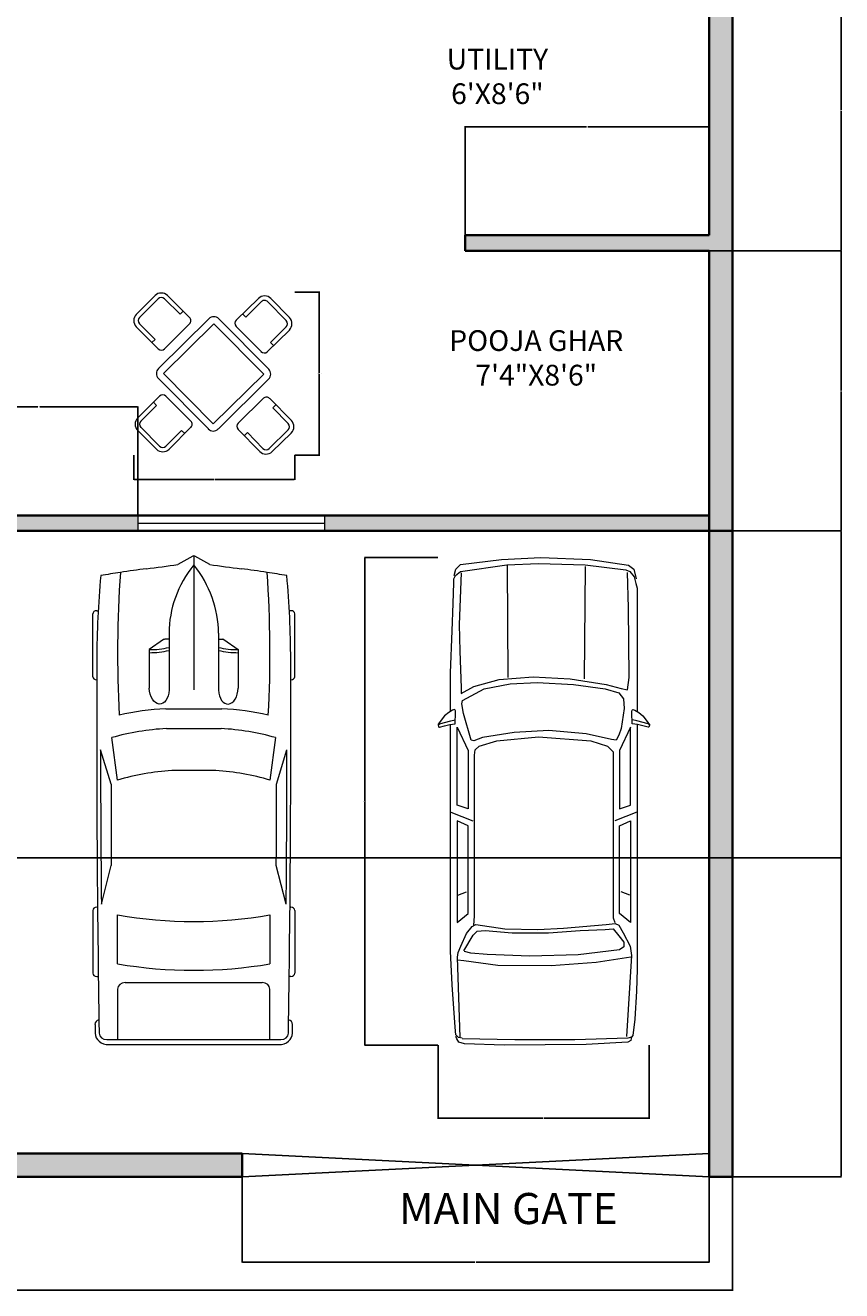
# Model space of a CAD drawing. Units: inches. Extents: x -89 to 661, y -827 to 77.
# Tile 3 of 5: x 347 to 661, y -827 to -339. Entities that reach past the tile are written whole.
import ezdxf

# ---------------------------------------------------------------- set-up
doc = ezdxf.new("R2010")
doc.units = ezdxf.units.IN
doc.header["$MEASUREMENT"] = 0
for name, color, linetype, lineweight in [('A-ANNO-DIMS', 2, 'Continuous', 18), ('A-ANNO-TEXT', 7, 'Continuous', 18), ('A-AREA-IDEN', 7, 'Continuous', 18), ('A-FURN', 34, 'Continuous', 18), ('A-GLAZ', 5, 'Continuous', 18), ('A-WALL', 7, 'Continuous', 35), ('A-WALL-PATT', 30, 'Continuous', 13), ('C-PRKG-VEHI', 5, 'Continuous', 13), ('L-GATE', 5, 'Continuous', 25)]:
    doc.layers.add(name, color=color, linetype=linetype, lineweight=lineweight)
doc.styles.get("Standard").update_dxf_attribs({"font": 'arial.ttf'})
doc.dimstyles.get("Standard").update_dxf_attribs({"dimtxt": 0.18, "dimasz": 0.18, "dimexe": 0.18, "dimexo": 0.0625, "dimgap": 0.09, "dimtad": 0, "dimtih": 1, "dimtoh": 1, "dimdec": 4, "dimzin": 0, "dimdsep": 46, "dimtxsty": 'Standard', "dimcen": 0.09, "dimadec": 0, "dimazin": 0, "dimtfac": 1, "dimtdec": 4, "dimtofl": 0, "dimtmove": 0, "dimatfit": 3, "dimfxl": 1, "dimtolj": 1, "dimtzin": 0, "dimarcsym": 0})

# ---------------------------------------------------------------- blocks, each defined once
blk = doc.blocks.new('*U2')
for p, q in [((21.1, 37.41), (21.1, 36.83)), ((46.55, 38.89), (22.35, 38.89)), ((47.8, 37.39), (47.8, 37.41)), ((87.99, 31.87), (74.76, 35.92)), ((134.31, 35.6), (119.29, 31.78)), ((135.45, 37.07), (135.45, 37.41)), ((136.7, 38.89), (160.9, 38.89)), ((162.15, 37.41), (162.15, 36.77)), ((70.03, 31.54), (86.41, 29.35)), ((138.42, 29.35), (157.25, 29.35)), ((186.47, 29.35), (167.01, 29.35)), ((186.47, -33.5), (186.47, 33.5)), ((188.4, -32.76), (188.4, 32.76)), ((164.52, 26.39), (164.52, -26.39)), ((32.27, 11.63), (36.13, 17.17)), ((36.13, 17.17), (50.94, 17.17)), ((32.12, 9.51), (32.12, 11.15)), ((58.92, -10.77), (58.92, 10.77)), ((66.55, -10.53), (66.55, 10.53)), ((186.47, -10.53), (186.47, 10.53)), ((3.27, 6.13), (0.1, 0.41)), ((29.77, 9.51), (51.68, 9.51)), ((82.74, 8.5), (82.74, -8.5)), ((0, 0), (51.68, 0)), ((0.1, -0.41), (3.27, -6.13)), ((29.77, -9.51), (51.68, -9.51)), ((32.12, -9.51), (32.12, -11.15)), ((32.27, -11.63), (36.13, -17.17)), ((36.13, -17.17), (50.94, -17.17)), ((86.41, -29.35), (70.03, -31.54)), ((87.99, -31.87), (74.76, -35.92)), ((134.31, -35.6), (119.29, -31.78)), ((157.25, -29.35), (138.42, -29.35)), ((167.01, -29.35), (186.47, -29.35)), ((21.1, -37.41), (21.1, -36.83)), ((46.55, -38.89), (22.35, -38.89)), ((47.8, -37.39), (47.8, -37.41)), ((135.45, -37.07), (135.45, -37.41)), ((136.7, -38.89), (160.9, -38.89)), ((162.15, -37.41), (162.15, -36.77))]:
    blk.add_line(p, q)
for centre, major_axis, ratio, start_param, end_param in [((266.03, -27.52), (0, 313.31), 0.842304, 1.367076, 1.39176), ((41.19, -490.86), (0, 528.23), 0.842304, 0.00281, 0.075598), ((22.35, 37.41), (0, -1.48), 0.842304, 3.141593, 4.712389), ((64.48, -10555.62), (0, 10593.03), 0.842304, -0.013397, 0.002797), ((46.55, 37.41), (0, 1.48), 0.842304, -1.570796, 0), ((64.48, -10555.62), (0, -10591.55), 0.842304, 3.133765, 3.140441), ((136.7, 37.41), (0, -1.48), 0.842304, 3.141593, 4.712389), ((160.9, 37.41), (0, 1.48), 0.842304, -1.570796, 0), ((180.63, 35.84), (0, 2.22), 0.842304, -0.013017, 1.249894), ((64.48, -10556.36), (0, 10595.31), 0.842304, -0.013397, -0.013017), ((183.98, 33.5), (0, -2.96), 0.842304, 1.570796, 3.128196), ((183.98, 32.76), (0, -5.25), 0.842304, 1.570796, 3.128196), ((37.47, -593.96), (0, -623.33), 0.842304, 3.096046, 3.200911), ((135.29, 5.39), (0, 81.77), 0.842304, 1.245306, 1.50788), ((149.6, 2.8), (0, -79.58), 0.842304, 4.372215, 4.640744), ((95.79, -3666.35), (0, -3698.24), 0.842304, 3.134049, 3.144098), ((17.08, 0), (0, 147.02), 0.842304, 4.511394, 4.913384), ((35.91, 0), (0, 147.02), 0.842304, 4.511394, 4.913384), ((167.01, 26.39), (0, 2.96), 0.842304, 0, 1.570796), ((259.18, -27.52), (0, -305.3), 0.842304, 4.528606, 4.561838), ((134.4, 5.39), (0, -89.78), 0.842304, 4.449482, 4.652344), ((-204.49, 52.4), (0, -250.96), 0.842304, 1.385369, 1.434372), ((13.04, 17.01), (0, 27.42), 0.842304, 4.435146, 4.718221), ((14.2, 17.01), (0, 27.42), 0.842304, 4.435146, 4.718221), ((50.79, 13.34), (6.34, -0.36), 0.603834, -1.395552, 1.581315), ((32.75, 11.15), (0, 0.74), 0.842304, 0.879714, 1.570796), ((29.77, -46.66), (0, 56.17), 0.842304, 0, 0.590319), ((0.62, 0), (0, -0.74), 0.842304, 4.131459, 5.293319), ((29.77, 46.66), (0, 56.17), 0.842304, 2.551274, 3.141593), ((-204.49, -52.4), (0, 250.96), 0.842304, -1.434372, -1.385369), ((13.04, -17.01), (0, -27.42), 0.842304, 1.564964, 1.848039), ((14.2, -17.01), (0, -27.42), 0.842304, 1.564964, 1.848039), ((149.6, -2.8), (0, -79.58), 0.842304, -1.499151, -1.230623), ((32.75, -11.15), (0, -0.74), 0.842304, 4.712389, 5.403472), ((134.4, -5.39), (0, -89.78), 0.842304, -1.510751, -1.307889), ((135.29, -5.39), (0, -81.77), 0.842304, -1.50788, -1.245306), ((259.18, 27.52), (0, 305.3), 0.842304, 1.721348, 1.754579), ((266.03, 27.52), (0, 313.31), 0.842304, 1.749832, 1.774517), ((37.47, 593.96), (0, -623.33), 0.842304, -0.059319, 0.045547), ((167.01, -26.39), (0, -2.96), 0.842304, 4.712389, 6.283185), ((95.79, 3666.35), (0, -3698.24), 0.842304, -0.002505, 0.007544), ((183.98, -33.5), (0, 2.96), 0.842304, 3.15499, 4.712389), ((183.98, -32.76), (0, -5.25), 0.842304, 0.013397, 1.570796), ((41.19, 490.86), (0, -528.23), 0.842304, -0.075598, -0.00281), ((22.35, -37.41), (0, 1.48), 0.842304, 1.570796, 3.141593), ((64.48, 10555.62), (0, 10593.03), 0.842304, 3.138796, 3.15499), ((46.55, -37.41), (0, -1.48), 0.842304, 0, 1.570796), ((64.48, 10555.62), (0, -10591.55), 0.842304, 0.001152, 0.007828), ((136.7, -37.41), (0, -1.48), 0.842304, -1.570796, 0), ((160.9, -37.41), (0, 1.48), 0.842304, 3.141593, 4.712389), ((180.63, -35.84), (0, -2.22), 0.842304, -1.249894, 0.013017), ((64.48, 10556.36), (0, 10595.31), 0.842304, 3.15461, 3.15499)]:
    blk.add_ellipse(centre, major_axis=major_axis, ratio=ratio, start_param=start_param, end_param=end_param)
at = {"extrusion": (0, 0, -1)}
blk.add_ellipse((50.79, -13.34), major_axis=(6.34, 0.36), ratio=0.603834, start_param=-1.395552, end_param=1.581315, dxfattribs=at)
blk = doc.blocks.new('A$C381B4D24')
for p, q in [((-0.244, 1.001), (-0.212, 1.042)), ((-0.212, 1.042), (-0.142, 1.096)), ((-0.133, 1.095), (-0.162, 0.981)), ((-0.142, 1.096), (-0.127, 1.108)), ((-0.12, 1.108), (-0.133, 1.095)), ((-0.127, 1.108), (-0.12, 1.108)), ((-0.11, 1.042), (-0.124, 0.989)), ((-0.119, 1.108), (-0.097, 1.101)), ((-0.097, 1.095), (-0.11, 1.042)), ((-0.097, 1.101), (-0.097, 1.095)), ((-1.777, 0.52), (-1.719, 0.898)), ((-1.719, 0.898), (-1.68, 0.953)), ((-1.68, 0.953), (-1.583, 0.977)), ((-1.672, 0.873), (-1.658, 0.914)), ((-1.658, 0.914), (-1.605, 0.955)), ((-1.293, 0.898), (-1.648, 0.89)), ((-1.605, 0.955), (-1.538, 0.971)), ((-1.538, 0.971), (-1.491, 0.987)), ((-1.491, 0.987), (-0.253, 0.987)), ((-0.596, 0.906), (-1.293, 0.898)), ((-0.473, 0.89), (-0.596, 0.906)), ((-0.486, 0.827), (-0.473, 0.89)), ((-0.274, 0.942), (-0.269, 0.963)), ((-0.269, 0.935), (-0.274, 0.942)), ((-0.269, 0.963), (-0.244, 1.001)), ((-0.263, 0.932), (-0.269, 0.935)), ((-0.246, 0.932), (-0.263, 0.932)), ((-0.131, 0.936), (-0.246, 0.932)), ((-0.162, 0.981), (-0.17, 0.938)), ((-0.128, 0.963), (-0.131, 0.936)), ((-0.124, 0.989), (-0.128, 0.963)), ((-0.124, 0.987), (2.324, 0.987)), ((0.682, 0.92), (-0.097, 0.92)), ((-0.097, 0.92), (0.136, 0.809)), ((0.721, 0.809), (0.682, 0.92)), ((0.753, 0.983), (0.838, 0.761)), ((0.838, 0.92), (1.857, 0.92)), ((0.89, 0.809), (0.838, 0.92)), ((1.585, 0.912), (1.552, 0.825)), ((1.857, 0.92), (1.766, 0.809)), ((1.961, 0.844), (2.095, 0.916)), ((2.095, 0.916), (2.188, 0.93)), ((2.188, 0.93), (2.998, 0.88)), ((2.206, 0.923), (2.258, 0.574)), ((2.324, 0.987), (2.546, 0.978)), ((2.546, 0.978), (2.826, 0.963)), ((2.826, 0.963), (2.989, 0.944)), ((2.989, 0.944), (3.007, 0.929)), ((2.998, 0.93), (3.039, 0.923)), ((3.007, 0.929), (3.015, 0.893)), ((3.015, 0.893), (3.033, 0.361)), ((3.039, 0.923), (3.056, 0.894)), ((3.056, 0.894), (3.08, 0.475)), ((-1.725, 0.465), (-1.672, 0.873)), ((-0.524, 0.677), (-0.486, 0.827)), ((-0.481, 0.666), (-0.442, 0.801)), ((-0.442, 0.801), (-0.383, 0.849)), ((-0.383, 0.849), (-0.286, 0.856)), ((-0.286, 0.856), (-0.085, 0.825)), ((-0.085, 0.825), (-0.019, 0.801)), ((-0.019, 0.801), (0.032, 0.777)), ((0.032, 0.777), (0.026, 0.73)), ((0.136, 0.809), (0.721, 0.809)), ((1.766, 0.809), (0.89, 0.809)), ((1.812, 0.746), (1.857, 0.761)), ((1.868, 0.766), (1.885, 0.802)), ((1.879, 0.674), (1.868, 0.766)), ((1.885, 0.802), (1.961, 0.844)), ((1.92, 0.745), (1.99, 0.802)), ((1.99, 0.802), (2.054, 0.852)), ((2.054, 0.852), (2.101, 0.852)), ((2.101, 0.852), (2.13, 0.809)), ((2.13, 0.809), (2.182, 0.396)), ((-0.583, 0.314), (-0.524, 0.677)), ((-0.526, 0.349), (-0.481, 0.666)), ((0.026, 0.73), (-0.033, 0.476)), ((0.039, 0.523), (0.091, 0.69)), ((0.091, 0.69), (0.149, 0.746)), ((0.149, 0.746), (1.812, 0.746)), ((1.914, 0.247), (1.879, 0.674)), ((1.926, 0.666), (1.92, 0.745)), ((1.938, 0.417), (1.926, 0.666)), ((-1.797, 0.023), (-1.777, 0.52)), ((0, 0), (0.039, 0.523)), ((2.258, 0.574), (2.293, 0.126)), ((-1.738, 0), (-1.725, 0.465)), ((-1.706, 0.464), (-0.583, 0.456)), ((-0.033, 0.476), (-0.065, 0.103)), ((1.961, 0.097), (1.938, 0.417)), ((2.182, 0.396), (2.194, -0.088)), ((3.08, 0.475), (3.085, -0.344)), ((-0.602, -0.056), (-0.583, 0.314)), ((-0.546, -0.016), (-0.526, 0.349)), ((3.033, 0.361), (3.033, -0.237)), ((1.926, -0.009), (1.914, 0.247)), ((-1.777, -0.371), (-1.797, 0.023)), ((-1.725, -0.318), (-1.738, 0)), ((-0.065, 0.103), (-0.046, -0.246)), ((0.039, -0.42), (0, 0)), ((1.961, -0.265), (1.961, 0.097)), ((2.293, 0.126), (2.287, -0.408)), ((-0.576, -0.395), (-0.602, -0.056)), ((-0.533, -0.286), (-0.546, -0.016)), ((1.92, -0.337), (1.926, -0.009)), ((2.194, -0.088), (2.177, -0.514)), ((-0.046, -0.246), (0.006, -0.563)), ((3.033, -0.237), (3.021, -0.764)), ((-1.726, -0.782), (-1.777, -0.371)), ((-1.658, -0.783), (-1.725, -0.318)), ((-1.719, -0.316), (-0.596, -0.308)), ((-0.481, -0.547), (-0.533, -0.286)), ((1.879, -0.628), (1.92, -0.337)), ((1.938, -0.536), (1.961, -0.265)), ((3.085, -0.344), (3.074, -0.742)), ((-0.505, -0.648), (-0.576, -0.395)), ((0.091, -0.595), (0.039, -0.42)), ((2.287, -0.408), (2.241, -0.749)), ((-0.364, -0.761), (-0.481, -0.547)), ((0.006, -0.563), (0.039, -0.65)), ((0.13, -0.634), (0.091, -0.595)), ((1.897, -0.664), (1.879, -0.628)), ((1.943, -0.614), (1.938, -0.536)), ((1.984, -0.657), (1.943, -0.614)), ((2.177, -0.514), (2.165, -0.678)), ((-0.434, -0.774), (-0.505, -0.648)), ((-0.234, -0.753), (-0.331, -0.769)), ((0.032, -0.674), (-0.234, -0.753)), ((-0.097, -0.817), (0.136, -0.706)), ((0.039, -0.65), (0.032, -0.674)), ((0.182, -0.642), (0.13, -0.634)), ((0.136, -0.706), (0.721, -0.706)), ((1.793, -0.642), (0.182, -0.642)), ((0.721, -0.706), (0.682, -0.817)), ((0.753, -0.88), (0.838, -0.658)), ((0.89, -0.706), (0.838, -0.817)), ((1.766, -0.706), (0.89, -0.706)), ((1.585, -0.809), (1.552, -0.722)), ((1.857, -0.817), (1.766, -0.706)), ((1.883, -0.65), (1.793, -0.642)), ((1.967, -0.721), (1.897, -0.664)), ((2.095, -0.778), (1.967, -0.721)), ((2.142, -0.749), (1.984, -0.657)), ((2.165, -0.678), (2.147, -0.742)), ((2.241, -0.749), (2.235, -0.813)), ((3.074, -0.742), (3.056, -0.799)), ((-1.68, -0.829), (-1.726, -0.782)), ((-1.616, -0.845), (-1.68, -0.829)), ((-1.618, -0.832), (-1.658, -0.783)), ((-1.642, -0.774), (-1.125, -0.797)), ((-1.585, -0.848), (-1.618, -0.832)), ((-1.545, -0.848), (-1.585, -0.848)), ((-1.338, -0.856), (-1.545, -0.848)), ((-1.064, -0.864), (-1.338, -0.856)), ((-1.125, -0.797), (-0.86, -0.789)), ((-0.643, -0.881), (-1.064, -0.864)), ((-0.86, -0.789), (-0.492, -0.774)), ((-0.397, -0.881), (-0.643, -0.881)), ((-0.492, -0.774), (-0.434, -0.774)), ((-0.256, -0.881), (-0.397, -0.881)), ((-0.331, -0.769), (-0.364, -0.761)), ((-0.269, -0.834), (-0.274, -0.841)), ((-0.274, -0.841), (-0.269, -0.862)), ((-0.263, -0.831), (-0.269, -0.834)), ((-0.269, -0.862), (-0.244, -0.9)), ((-0.246, -0.831), (-0.263, -0.831)), ((-0.131, -0.835), (-0.246, -0.831)), ((-0.162, -0.88), (-0.17, -0.837)), ((-0.133, -0.994), (-0.162, -0.88)), ((-0.128, -0.862), (-0.131, -0.835)), ((-0.124, -0.889), (-0.128, -0.862)), ((1.703, -0.881), (-0.125, -0.881)), ((0.682, -0.817), (-0.097, -0.817)), ((0.838, -0.817), (1.857, -0.817)), ((2.144, -0.881), (1.703, -0.881)), ((2.159, -0.806), (2.095, -0.778)), ((2.483, -0.864), (2.144, -0.881)), ((2.206, -0.813), (2.159, -0.806)), ((3.01, -0.785), (2.206, -0.813)), ((2.907, -0.837), (2.483, -0.864)), ((2.981, -0.829), (2.907, -0.837)), ((3.01, -0.803), (2.981, -0.829)), ((3.021, -0.82), (2.998, -0.828)), ((3.017, -0.764), (3.01, -0.803)), ((3.056, -0.799), (3.021, -0.82)), ((-0.244, -0.9), (-0.212, -0.941)), ((-0.212, -0.941), (-0.142, -0.995)), ((-0.142, -0.995), (-0.127, -1.007)), ((-0.12, -1.007), (-0.133, -0.994)), ((-0.127, -1.007), (-0.12, -1.007)), ((-0.11, -0.941), (-0.124, -0.889)), ((-0.119, -1.007), (-0.097, -1)), ((-0.097, -0.994), (-0.11, -0.941)), ((-0.097, -1), (-0.097, -0.994))]:
    blk.add_line(p, q)
blk = doc.blocks.new('A$C14754BF6')
for p, q in [((0.026, 1.576), (0.238, 1.789)), ((0.061, 1.541), (0.273, 1.753)), ((0.521, 1.577), (0.344, 1.753)), ((0.627, 1.541), (0.379, 1.789)), ((1.155, 1.511), (1.405, 1.756)), ((1.262, 1.546), (1.44, 1.721)), ((1.721, 1.506), (1.511, 1.72)), ((1.757, 1.541), (1.547, 1.755)), ((0.521, 1.577), (0.556, 1.612)), ((1.262, 1.546), (1.227, 1.581)), ((0.274, 1.188), (0.026, 1.435)), ((0.238, 1.294), (0.061, 1.47)), ((0.845, 1.527), (0.277, 0.964)), ((0.902, 1.47), (0.333, 0.907)), ((0.344, 1.188), (0.627, 1.471)), ((0.902, 1.47), (1.465, 0.901)), ((0.959, 1.526), (1.522, 0.958)), ((1.435, 1.155), (1.155, 1.441)), ((1.542, 1.26), (1.72, 1.435)), ((0.203, 1.258), (0.238, 1.294)), ((1.505, 1.154), (1.755, 1.399)), ((1.577, 1.224), (1.542, 1.26)), ((0.333, 0.907), (0.896, 0.338)), ((1.465, 0.901), (0.896, 0.338)), ((0.277, 0.85), (0.84, 0.282)), ((1.521, 0.845), (0.953, 0.282)), ((0.289, 0.653), (0.042, 0.406)), ((0.254, 0.547), (0.219, 0.583)), ((0.643, 0.371), (0.36, 0.653)), ((1.177, 0.348), (1.462, 0.628)), ((1.533, 0.627), (1.778, 0.377)), ((0.254, 0.547), (0.077, 0.37)), ((1.567, 0.52), (1.603, 0.555)), ((1.567, 0.52), (1.742, 0.342)), ((0.29, 0.088), (0.077, 0.3)), ((0.643, 0.3), (0.396, 0.052)), ((0.254, 0.052), (0.042, 0.264)), ((0.537, 0.265), (0.361, 0.088)), ((0.573, 0.229), (0.537, 0.265)), ((1.176, 0.277), (1.421, 0.027)), ((1.246, 0.205), (1.282, 0.24)), ((1.282, 0.24), (1.457, 0.062)), ((1.527, 0.061), (1.742, 0.271)), ((1.562, 0.025), (1.777, 0.235))]:
    blk.add_line(p, q)
for centre, radius, start, end in [((0.309, 1.718), 0.1, 45.0454, 135.0454), ((0.309, 1.718), 0.05, 45.0454, 135.0454), ((1.475, 1.685), 0.1, 44.4208, 134.4208), ((1.475, 1.685), 0.05, 44.4208, 134.4208), ((0.097, 1.506), 0.1, 135.0454, 225.0454), ((0.097, 1.506), 0.05, 135.0454, 225.0454), ((0.592, 1.506), 0.05, 315.0454, 45.0454), ((0.902, 1.47), 0.08, 44.7331, 134.7331), ((1.19, 1.476), 0.05, 134.4208, 224.4208), ((1.685, 1.471), 0.05, 314.4208, 44.4208), ((1.685, 1.471), 0.1, 314.4208, 44.4208), ((0.309, 1.223), 0.05, 225.0454, 315.0454), ((1.47, 1.19), 0.05, 224.4208, 314.4208), ((0.333, 0.907), 0.08, 134.7331, 224.7331), ((1.465, 0.901), 0.08, 314.7331, 44.7331), ((0.325, 0.618), 0.05, 45.0454, 135.0454), ((1.497, 0.592), 0.05, 44.4208, 134.4208), ((0.113, 0.335), 0.1, 135.0454, 225.0454), ((0.113, 0.335), 0.05, 135.0454, 225.0454), ((0.608, 0.335), 0.05, 315.0454, 45.0454), ((1.212, 0.312), 0.05, 134.4208, 224.4208), ((1.707, 0.307), 0.05, 314.4208, 44.4208), ((1.707, 0.307), 0.1, 314.4208, 44.4208), ((0.896, 0.338), 0.08, 224.7331, 314.7331), ((0.325, 0.123), 0.1, 225.0454, 315.0454), ((0.325, 0.123), 0.05, 225.0454, 315.0454), ((1.492, 0.097), 0.1, 224.4208, 314.4208), ((1.492, 0.097), 0.05, 224.4208, 314.4208)]:
    blk.add_arc(centre, radius, start, end)
blk = doc.blocks.new('WIN-72-NOM')
for p, q in [((0, 6), (0, 0)), ((0, 6), (71.86, 6)), ((71.86, 6), (71.86, 0)), ((0, 3), (71.86, 3)), ((0, 0), (71.86, 0))]:
    blk.add_line(p, q)
blk = doc.blocks.new('*D23')
at = {"layer": 'A-ANNO-DIMS', "color": 0, "lineweight": -2, "transparency": 16777216}
for p, q in [((505.67, -544.19), (477.36, -544.19)), ((477.54, -544.37), (477.54, -638)), ((477.54, -732), (477.54, -638.37)), ((505.67, -732.18), (477.36, -732.18))]:
    blk.add_line(p, q, dxfattribs=at)
at = {"layer": 'A-ANNO-DIMS', "color": 0, "transparency": 16777216}
for points in [[(477.51, -544.37), (477.57, -544.37), (477.54, -544.19)], [(477.51, -732), (477.57, -732), (477.54, -732.18)]]:
    blk.add_solid(points, dxfattribs=at)
at = {"layer": 'Defpoints', "color": 0, "transparency": 16777216}
for p in [(505.73, -544.19), (477.54, -732.18), (505.73, -732.18)]:
    blk.add_point(p, dxfattribs=at)
at = {"layer": 'A-ANNO-DIMS', "color": 0, "transparency": 16777216, "insert": (477.54, -638.18), "char_height": 0.18, "attachment_point": 5}
blk.add_mtext('\\A1;CAR 188', dxfattribs=at)
blk = doc.blocks.new('*D24')
at = {"layer": 'A-ANNO-DIMS', "color": 0, "lineweight": -2, "transparency": 16777216}
for p, q in [((505.73, -732.24), (505.73, -760.55)), ((587.13, -732.24), (587.13, -760.55)), ((505.91, -760.37), (546.23, -760.37)), ((586.95, -760.37), (546.64, -760.37))]:
    blk.add_line(p, q, dxfattribs=at)
at = {"layer": 'A-ANNO-DIMS', "color": 0, "transparency": 16777216}
for points in [[(505.91, -760.34), (505.91, -760.4), (505.73, -760.37)], [(586.95, -760.34), (586.95, -760.4), (587.13, -760.37)]]:
    blk.add_solid(points, dxfattribs=at)
at = {"layer": 'Defpoints', "color": 0, "transparency": 16777216}
for p in [(505.73, -732.18), (587.13, -732.18), (587.13, -760.37)]:
    blk.add_point(p, dxfattribs=at)
at = {"layer": 'A-ANNO-DIMS', "color": 0, "transparency": 16777216, "insert": (546.43, -760.37), "char_height": 0.18, "attachment_point": 5}
blk.add_mtext('\\A1;81', dxfattribs=at)
blk = doc.blocks.new('*D27')
at = {"layer": 'A-ANNO-DIMS', "color": 0, "lineweight": -2, "transparency": 16777216}
for p, q in [((450.59, -441.87), (460.12, -441.87)), ((459.94, -442.05), (459.94, -473.09)), ((459.94, -504.49), (459.94, -473.46)), ((450.59, -504.67), (460.12, -504.67))]:
    blk.add_line(p, q, dxfattribs=at)
at = {"layer": 'A-ANNO-DIMS', "color": 0, "transparency": 16777216}
for points in [[(459.91, -442.05), (459.97, -442.05), (459.94, -441.87)], [(459.91, -504.49), (459.97, -504.49), (459.94, -504.67)]]:
    blk.add_solid(points, dxfattribs=at)
at = {"layer": 'Defpoints', "color": 0, "transparency": 16777216}
for p in [(450.52, -441.87), (459.94, -441.87), (450.52, -504.67)]:
    blk.add_point(p, dxfattribs=at)
at = {"layer": 'A-ANNO-DIMS', "color": 0, "transparency": 16777216, "insert": (459.94, -473.27), "char_height": 0.18, "attachment_point": 5}
blk.add_mtext('\\A1;TABLE SET 63', dxfattribs=at)
blk = doc.blocks.new('*D28')
at = {"layer": 'A-ANNO-DIMS', "color": 0, "lineweight": -2, "transparency": 16777216}
for p, q in [((388.44, -504.73), (388.44, -514.27)), ((450.52, -504.73), (450.52, -514.27)), ((388.62, -514.09), (419.26, -514.09)), ((450.34, -514.09), (419.7, -514.09))]:
    blk.add_line(p, q, dxfattribs=at)
at = {"layer": 'A-ANNO-DIMS', "color": 0, "transparency": 16777216}
for points in [[(388.62, -514.06), (388.62, -514.12), (388.44, -514.09)], [(450.34, -514.06), (450.34, -514.12), (450.52, -514.09)]]:
    blk.add_solid(points, dxfattribs=at)
at = {"layer": 'Defpoints', "color": 0, "transparency": 16777216}
for p in [(388.44, -504.67), (450.52, -504.67), (450.52, -514.09)]:
    blk.add_point(p, dxfattribs=at)
at = {"layer": 'A-ANNO-DIMS', "color": 0, "transparency": 16777216, "insert": (419.48, -514.09), "char_height": 0.18, "attachment_point": 5}
blk.add_mtext('\\A1;62', dxfattribs=at)
blk = doc.blocks.new('*D31')
at = {"layer": 'A-ANNO-DIMS', "color": 0, "lineweight": -2, "transparency": 16777216}
for p, q in [((-1.81, -783), (-1.81, -826.85)), ((619.19, -783), (619.19, -826.85)), ((-1.63, -826.67), (308.41, -826.67)), ((619.01, -826.67), (308.96, -826.67))]:
    blk.add_line(p, q, dxfattribs=at)
at = {"layer": 'A-ANNO-DIMS', "color": 0, "transparency": 16777216}
for points in [[(-1.63, -826.64), (-1.63, -826.7), (-1.81, -826.67)], [(619.01, -826.64), (619.01, -826.7), (619.19, -826.67)]]:
    blk.add_solid(points, dxfattribs=at)
at = {"layer": 'Defpoints', "color": 0, "transparency": 16777216}
for p in [(-1.81, -782.94), (619.19, -782.94), (619.19, -826.67)]:
    blk.add_point(p, dxfattribs=at)
at = {"layer": 'A-ANNO-DIMS', "color": 0, "transparency": 16777216, "insert": (308.69, -826.67), "char_height": 0.18, "attachment_point": 5}
blk.add_mtext('\\A1;621', dxfattribs=at)
blk = doc.blocks.new('*D37')
at = {"layer": 'A-ANNO-DIMS', "color": 0, "lineweight": -2, "transparency": 16777216}
for p, q in [((610.25, -317.94), (661.23, -317.94)), ((661.05, -318.12), (661.05, -371.76)), ((661.05, -425.76), (661.05, -372.12)), ((610.25, -425.94), (661.23, -425.94))]:
    blk.add_line(p, q, dxfattribs=at)
at = {"layer": 'A-ANNO-DIMS', "color": 0, "transparency": 16777216}
for points in [[(661.02, -318.12), (661.08, -318.12), (661.05, -317.94)], [(661.02, -425.76), (661.08, -425.76), (661.05, -425.94)]]:
    blk.add_solid(points, dxfattribs=at)
at = {"layer": 'Defpoints', "color": 0, "transparency": 16777216}
for p in [(610.19, -317.94), (661.05, -317.94), (610.19, -425.94)]:
    blk.add_point(p, dxfattribs=at)
at = {"layer": 'A-ANNO-DIMS', "color": 0, "transparency": 16777216, "insert": (661.05, -371.94), "char_height": 0.18, "attachment_point": 5}
blk.add_mtext('\\A1;108', dxfattribs=at)
blk = doc.blocks.new('*D38')
at = {"layer": 'A-ANNO-DIMS', "color": 0, "lineweight": -2, "transparency": 16777216}
for p, q in [((610.25, -425.94), (661.23, -425.94)), ((661.05, -426.12), (661.05, -479.76)), ((661.05, -533.76), (661.05, -480.12)), ((619.25, -533.94), (661.23, -533.94))]:
    blk.add_line(p, q, dxfattribs=at)
at = {"layer": 'A-ANNO-DIMS', "color": 0, "transparency": 16777216}
for points in [[(661.02, -426.12), (661.08, -426.12), (661.05, -425.94)], [(661.02, -533.76), (661.08, -533.76), (661.05, -533.94)]]:
    blk.add_solid(points, dxfattribs=at)
at = {"layer": 'Defpoints', "color": 0, "transparency": 16777216}
for p in [(610.19, -425.94), (661.05, -425.94), (619.19, -533.94)]:
    blk.add_point(p, dxfattribs=at)
at = {"layer": 'A-ANNO-DIMS', "color": 0, "transparency": 16777216, "insert": (661.05, -479.94), "char_height": 0.18, "attachment_point": 5}
blk.add_mtext('\\A1;108', dxfattribs=at)
blk = doc.blocks.new('*D39')
at = {"layer": 'A-ANNO-DIMS', "color": 0, "lineweight": -2, "transparency": 16777216}
for p, q in [((619.25, -533.94), (661.23, -533.94)), ((661.05, -534.12), (661.05, -658.26)), ((661.05, -782.76), (661.05, -658.62)), ((619.25, -782.94), (661.23, -782.94))]:
    blk.add_line(p, q, dxfattribs=at)
at = {"layer": 'A-ANNO-DIMS', "color": 0, "transparency": 16777216}
for points in [[(661.02, -534.12), (661.08, -534.12), (661.05, -533.94)], [(661.02, -782.76), (661.08, -782.76), (661.05, -782.94)]]:
    blk.add_solid(points, dxfattribs=at)
at = {"layer": 'Defpoints', "color": 0, "transparency": 16777216}
for p in [(619.19, -533.94), (661.05, -533.94), (619.19, -782.94)]:
    blk.add_point(p, dxfattribs=at)
at = {"layer": 'A-ANNO-DIMS', "color": 0, "transparency": 16777216, "insert": (661.05, -658.44), "char_height": 0.18, "attachment_point": 5}
blk.add_mtext('\\A1;249', dxfattribs=at)
blk = doc.blocks.new('*D40')
at = {"layer": 'A-ANNO-DIMS', "color": 0, "lineweight": -2, "transparency": 16777216}
for p, q in [((430.19, -774), (430.19, -815.98)), ((610.19, -774), (610.19, -815.98)), ((430.37, -815.8), (519.91, -815.8)), ((610.01, -815.8), (520.47, -815.8))]:
    blk.add_line(p, q, dxfattribs=at)
at = {"layer": 'A-ANNO-DIMS', "color": 0, "transparency": 16777216}
for points in [[(430.37, -815.77), (430.37, -815.83), (430.19, -815.8)], [(610.01, -815.77), (610.01, -815.83), (610.19, -815.8)]]:
    blk.add_solid(points, dxfattribs=at)
at = {"layer": 'Defpoints', "color": 0, "transparency": 16777216}
for p in [(430.19, -773.94), (610.19, -773.94), (430.19, -815.8)]:
    blk.add_point(p, dxfattribs=at)
at = {"layer": 'A-ANNO-DIMS', "color": 0, "transparency": 16777216, "insert": (520.19, -815.8), "char_height": 0.18, "attachment_point": 5}
blk.add_mtext('\\A1;180', dxfattribs=at)
blk = doc.blocks.new('*D60')
at = {"layer": 'A-ANNO-DIMS', "color": 0, "lineweight": -2, "transparency": 16777216}
for p, q in [((334.85, -533.94), (661.23, -533.94)), ((661.05, -534.12), (661.05, -596.76)), ((661.05, -659.76), (661.05, -597.12)), ((334.85, -659.94), (661.23, -659.94))]:
    blk.add_line(p, q, dxfattribs=at)
at = {"layer": 'A-ANNO-DIMS', "color": 0, "transparency": 16777216}
for points in [[(661.02, -534.12), (661.08, -534.12), (661.05, -533.94)], [(661.02, -659.76), (661.08, -659.76), (661.05, -659.94)]]:
    blk.add_solid(points, dxfattribs=at)
at = {"layer": 'Defpoints', "color": 0, "transparency": 16777216}
for p in [(334.79, -533.94), (661.05, -533.94), (334.79, -659.94)]:
    blk.add_point(p, dxfattribs=at)
at = {"layer": 'A-ANNO-DIMS', "color": 0, "transparency": 16777216, "insert": (661.05, -596.94), "char_height": 0.18, "attachment_point": 5}
blk.add_mtext('\\A1;126', dxfattribs=at)
blk = doc.blocks.new('*D73')
at = {"layer": 'A-ANNO-DIMS', "color": 0, "lineweight": -2, "transparency": 16777216}
for p, q in [((516.19, -419.88), (516.19, -377.9)), ((516.37, -378.08), (562.97, -378.08)), ((610.01, -378.08), (563.4, -378.08)), ((610.19, -419.88), (610.19, -377.9))]:
    blk.add_line(p, q, dxfattribs=at)
at = {"layer": 'A-ANNO-DIMS', "color": 0, "transparency": 16777216}
for points in [[(516.37, -378.05), (516.37, -378.11), (516.19, -378.08)], [(610.01, -378.05), (610.01, -378.11), (610.19, -378.08)]]:
    blk.add_solid(points, dxfattribs=at)
at = {"layer": 'Defpoints', "color": 0, "transparency": 16777216}
for p in [(610.19, -378.08), (516.19, -419.94), (610.19, -419.94)]:
    blk.add_point(p, dxfattribs=at)
at = {"layer": 'A-ANNO-DIMS', "color": 0, "transparency": 16777216, "insert": (563.19, -378.08), "char_height": 0.18, "attachment_point": 5}
blk.add_mtext('\\A1;94', dxfattribs=at)
blk = doc.blocks.new('*D74')
at = {"layer": 'A-ANNO-DIMS', "color": 0, "lineweight": -2, "transparency": 16777216}
for p, q in [((313.68, -527.88), (313.68, -485.9)), ((313.86, -486.08), (351.48, -486.08)), ((389.89, -486.08), (352.27, -486.08)), ((390.07, -527.88), (390.07, -485.9))]:
    blk.add_line(p, q, dxfattribs=at)
at = {"layer": 'A-ANNO-DIMS', "color": 0, "transparency": 16777216}
for points in [[(313.86, -486.05), (313.86, -486.11), (313.68, -486.08)], [(389.89, -486.05), (389.89, -486.11), (390.07, -486.08)]]:
    blk.add_solid(points, dxfattribs=at)
at = {"layer": 'Defpoints', "color": 0, "transparency": 16777216}
for p in [(390.07, -486.08), (313.68, -527.94), (390.07, -527.94)]:
    blk.add_point(p, dxfattribs=at)
at = {"layer": 'A-ANNO-DIMS', "color": 0, "transparency": 16777216, "insert": (351.88, -486.08), "char_height": 0.18, "attachment_point": 5}
blk.add_mtext('\\A1;76.39', dxfattribs=at)

msp = doc.modelspace()

# ---------------------------------------------------------------- hatches: boundary and pattern name
at = {"layer": 'A-WALL-PATT'}
h = msp.add_hatch(color=256, dxfattribs=at)
h.dxf.hatch_style = 1
h.paths.add_polyline_path([(255.186, 29.06), (-1.814, 29.06), (-1.814, -33.94), (7.186, -33.94), (7.186, -27.94), (7.186, 20.06), (255.186, 20.06)])
h.paths.add_polyline_path([(174.616, -27.94), (7.186, -27.94), (7.186, -33.94), (174.616, -33.94)], flags=17)
h.paths.add_polyline_path([(7.186, -33.94), (-1.814, -33.94), (-1.814, -527.94), (7.186, -527.94), (7.186, -425.94), (7.186, -311.94), (7.186, -207.94)])
h.paths.add_polyline_path([(7.186, -527.94), (-1.814, -527.94), (-1.814, -782.94), (430.186, -782.94), (430.186, -773.94), (7.186, -773.94)])
h = msp.add_hatch(color=256, dxfattribs=at)
h.dxf.hatch_style = 1
h.paths.add_polyline_path([(619.186, 29.06), (417.186, 29.06), (417.186, 20.06), (610.186, 20.06), (610.186, -142.94), (610.186, -311.94), (610.186, -419.94), (516.186, -419.94), (516.186, -425.94), (610.186, -425.94), (610.186, -527.94), (610.186, -533.94), (619.186, -533.94)])
h = msp.add_hatch(color=256, dxfattribs=at)
h.dxf.hatch_style = 1
h.paths.add_polyline_path([(619.186, -533.94), (610.186, -533.94), (610.186, -773.94), (610.186, -782.94), (619.186, -782.94)])
h.paths.add_polyline_path([(610.186, -527.94), (461.934, -527.94), (461.934, -533.94), (610.186, -533.94)])
h.paths.add_polyline_path([(390.071, -527.94), (313.682, -527.94), (313.682, -528.84), (313.682, -533.94), (390.071, -533.94)])
h.paths.add_polyline_path([(334.788, -533.94), (328.788, -533.94), (328.788, -653.94), (334.788, -653.94)])
h.paths.add_polyline_path([(334.788, -653.94), (226.788, -653.94), (226.788, -659.94), (334.788, -659.94)])
h.paths.add_polyline_path([(232.788, -533.94), (226.788, -533.94), (226.788, -573.94), (226.788, -653.94), (232.788, -653.94)])
h.paths.add_polyline_path([(245.682, -528.84), (245.682, -527.94), (226.788, -527.94), (226.788, -533.94), (232.788, -533.94), (245.682, -533.94)])
h.paths.add_polyline_path([(226.788, -629.94), (184.634, -629.94), (184.634, -635.94), (226.788, -635.94)])
h.paths.add_polyline_path([(76.788, -533.94), (70.788, -533.94), (70.788, -635.94), (112.77, -635.94), (112.77, -629.94), (76.788, -629.94)])
h.paths.add_polyline_path([(186.788, -527.94), (55.963, -527.94), (55.963, -533.94), (186.788, -533.94)])
h.paths.add_polyline_path([(17.901, -527.94), (7.186, -527.94), (7.186, -533.94), (17.901, -533.94)])

# ---------------------------------------------------------------- linework, layer by layer
at = {"layer": 'A-WALL'}
for p, q in [((619.186, 29.06), (619.186, -782.94)), ((610.186, -311.94), (610.186, -419.94)), ((516.186, -419.94), (610.186, -419.94)), ((516.186, -419.94), (516.186, -425.94)), ((516.186, -425.94), (610.186, -425.94)), ((610.186, -425.94), (610.186, -527.94)), ((313.682, -527.94), (610.186, -527.94)), ((610.186, -527.94), (610.186, -773.94)), ((313.682, -533.94), (619.186, -533.94)), ((7.186, -773.94), (430.186, -773.94)), ((430.186, -773.94), (430.186, -782.94)), ((610.186, -773.94), (610.186, -782.94)), ((-1.814, -782.94), (430.186, -782.94)), ((610.186, -782.94), (619.186, -782.94))]:
    msp.add_line(p, q, dxfattribs=at)
at = {"layer": 'L-GATE'}
for p, q in [((430.186, -782.94), (610.186, -773.94)), ((610.186, -782.94), (430.186, -773.94))]:
    msp.add_line(p, q, dxfattribs=at)

# ---------------------------------------------------------------- block references
at = {"layer": 'A-FURN', "xscale": 34.11172618751257, "yscale": 34.11172618751257, "zscale": 34.11172618751257}
msp.add_blockref('A$C14754BF6', (388.553, -504.221), dxfattribs=at)
at = {"layer": 'A-GLAZ'}
msp.add_blockref('WIN-72-NOM', (390.071, -533.94), dxfattribs=at)
at = {"layer": 'C-PRKG-VEHI', "rotation": 270}
msp.add_blockref('*U2', (411.592, -543.577), dxfattribs=at)
at = {"layer": 'C-PRKG-VEHI', "xscale": 38.50453824810685, "yscale": 38.50453824810685, "zscale": 38.50453824810685, "rotation": 270}
msp.add_blockref('A$C381B4D24', (544.49, -613.374), dxfattribs=at)

# ---------------------------------------------------------------- texts
at = {"layer": 'A-ANNO-TEXT', "insert": (473.495, -789.177), "char_height": 12, "attachment_point": 1}
msp.add_mtext_dynamic_manual_height_columns('\\pxqc;{\\fArial|b1|i0|c0|p34;MAIN GATE}', width=118.5848, gutter_width=1, heights=[0], dxfattribs=at)
at = {"layer": 'A-AREA-IDEN', "char_height": 8, "attachment_point": 1}
for s, width, insert in [('\\pxqc;UTILITY\\P6\'X8\'6"', 56.29646, (500.443, -348.041)), ('\\pxqc;POOJA GHAR\\P7\'4"X8\'6"', 76.33891, (505.392, -456.549))]:
    msp.add_mtext_dynamic_manual_height_columns(s, width=width, gutter_width=1, heights=[0], dxfattribs=dict(at, insert=insert))

# ---------------------------------------------------------------- dimensions: what is measured, and where the dimension line sits
at = {"layer": 'A-ANNO-DIMS'}
for base, p1, p2, angle, picture, middle in [((661.046, -317.94), (610.186, -425.94), (610.186, -317.94), 90, '*D37', (661.046, -371.94)), ((661.046, -425.94), (619.186, -533.94), (610.186, -425.94), 90, '*D38', (661.046, -479.94)), ((661.046, -533.94), (334.788, -659.94), (334.788, -533.94), 90, '*D60', (661.046, -596.94)), ((661.046, -533.94), (619.186, -782.94), (619.186, -533.94), 90, '*D39', (661.046, -658.44)), ((430.186, -815.8), (610.186, -773.94), (430.186, -773.94), 180, '*D40', (520.186, -815.8))]:
    dim = msp.add_linear_dim(base=base, p1=p1, p2=p2, angle=angle, dimstyle='Standard', override={"dimdec": 0, "dimlfac": 1, "dimrnd": 0, "dimzin": 0, "dimdsep": 46, "dimlunit": 2}, dxfattribs=at)
    dim.commit()
    dim.dimension.update_dxf_attribs({"geometry": picture, "text_midpoint": middle})
for base, p1, p2, override, picture, middle in [((610.186, -378.08), (516.186, -419.94), (610.186, -419.94), {"dimdec": 0, "dimlfac": 1, "dimrnd": 0, "dimzin": 0, "dimdsep": 46, "dimlunit": 2}, '*D73', (563.186, -378.08)), ((390.071, -486.08), (313.682, -527.94), (390.071, -527.94), {"dimdec": 2, "dimlfac": 1, "dimrnd": 0, "dimzin": 0, "dimdsep": 46, "dimlunit": 2}, '*D74', (351.876, -486.08)), ((450.523, -514.092), (388.437, -504.672), (450.523, -504.672), {"dimdec": 0, "dimlfac": 1, "dimrnd": 0, "dimzin": 0, "dimdsep": 46, "dimlunit": 2}, '*D28', (419.48, -514.092)), ((587.134, -760.374), (505.733, -732.177), (587.134, -732.177), {"dimdec": 0, "dimlfac": 1, "dimrnd": 0, "dimzin": 0, "dimdsep": 46, "dimlunit": 2}, '*D24', (546.433, -760.374)), ((619.186, -826.669), (-1.814, -782.94), (619.186, -782.94), {"dimdec": 0, "dimlfac": 1, "dimrnd": 0, "dimzin": 0, "dimdsep": 46, "dimlunit": 2}, '*D31', (308.686, -826.669))]:
    dim = msp.add_linear_dim(base=base, p1=p1, p2=p2, dimstyle='Standard', override=override, dxfattribs=at)
    dim.commit()
    dim.dimension.update_dxf_attribs({"geometry": picture, "text_midpoint": middle})
for base, p1, p2, angle, text, picture, middle in [((459.943, -441.874), (450.523, -504.672), (450.523, -441.874), 90, 'TABLE SET <>', '*D27', (459.943, -473.273)), ((477.535, -732.177), (505.733, -544.193), (505.733, -732.177), 270, 'CAR <>', '*D23', (477.535, -638.185))]:
    dim = msp.add_linear_dim(base=base, p1=p1, p2=p2, angle=angle, text=text, dimstyle='Standard', override={"dimdec": 0, "dimlfac": 1, "dimrnd": 0, "dimzin": 0, "dimdsep": 46, "dimlunit": 2}, dxfattribs=at)
    dim.commit()
    dim.dimension.update_dxf_attribs({"geometry": picture, "text_midpoint": middle})

doc.saveas('drawing.dxf')
